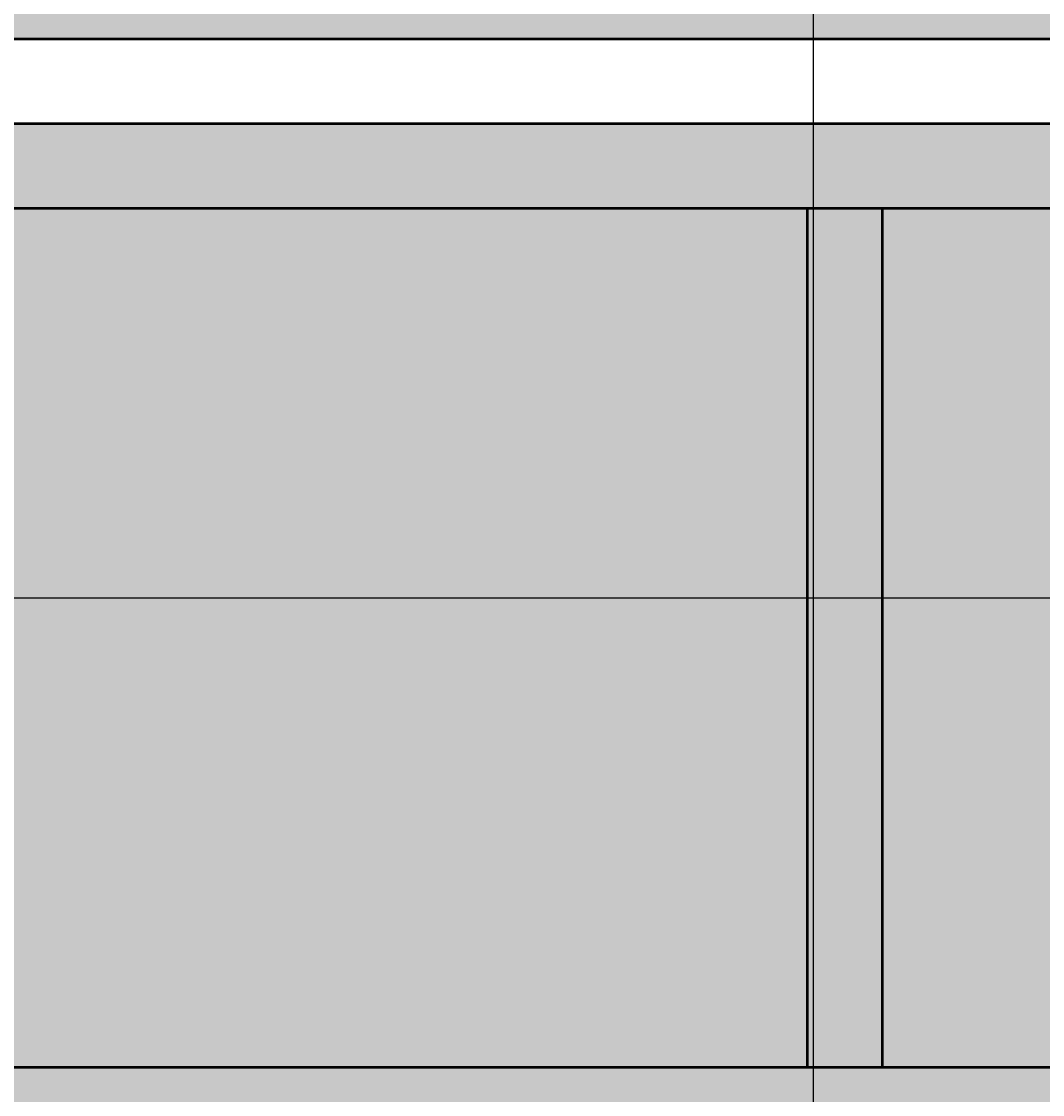
# Model space of a CAD drawing. Units: inches. Extents: x -12 to 334, y -10 to 186.
# Tile 52 of 77: x 198 to 222, y 69 to 94. Entities that reach past the tile are written whole.
import ezdxf

# ---------------------------------------------------------------- set-up
doc = ezdxf.new("R2010")
doc.units = ezdxf.units.IN
doc.header["$MEASUREMENT"] = 0
for name, color, linetype, lineweight in [('M-DIMS', 2, 'Continuous', 18), ('M-EQPM', 7, 'Continuous', 50), ('M-EQPM-PATT', 8, 'Continuous', 18)]:
    doc.layers.add(name, color=color, linetype=linetype, lineweight=lineweight)
doc.styles.get("Standard").update_dxf_attribs({"font": 'arial.ttf'})
doc.dimstyles.get("Standard").update_dxf_attribs({"dimtxt": 0.18, "dimasz": 0.18, "dimexe": 0.18, "dimexo": 0.0625, "dimgap": 0.09, "dimtad": 0, "dimtih": 1, "dimtoh": 1, "dimdec": 4, "dimzin": 0, "dimdsep": 46, "dimtxsty": 'Standard', "dimcen": 0.09, "dimadec": 0, "dimazin": 0, "dimtfac": 1, "dimtdec": 4, "dimtofl": 0, "dimtmove": 0, "dimatfit": 3, "dimfxl": 1, "dimtolj": 1, "dimtzin": 0, "dimarcsym": 0})

# ---------------------------------------------------------------- blocks, each defined once
blk = doc.blocks.new('*D1')
at = {"layer": 'Defpoints', "color": 0, "transparency": 16777216}
for p in [(281.426, 91.899), (3.376, 80.692), (281.426, 14.304)]:
    blk.add_point(p, dxfattribs=at)
at = {"layer": 'M-DIMS', "color": 0, "lineweight": -2, "transparency": 16777216}
for p, q in [((281.426, 91.836), (281.426, 14.124)), ((3.376, 80.629), (3.376, 14.124)), ((3.556, 14.304), (141.935, 14.304)), ((281.246, 14.304), (142.867, 14.304))]:
    blk.add_line(p, q, dxfattribs=at)
at = {"layer": 'M-DIMS', "color": 0, "transparency": 16777216}
for points in [[(3.556, 14.334), (3.556, 14.274), (3.376, 14.304)], [(281.246, 14.334), (281.246, 14.274), (281.426, 14.304)]]:
    blk.add_solid(points, dxfattribs=at)
at = {"layer": 'M-DIMS', "color": 0, "transparency": 16777216, "insert": (142.401, 14.304), "char_height": 0.18, "attachment_point": 5}
blk.add_mtext('\\A1;278.05', dxfattribs=at)
blk = doc.blocks.new('*D17')
at = {"layer": 'Defpoints', "color": 0, "transparency": 16777216}
for p in [(106.177, 102.896), (105.892, 56.321), (295.976, 56.321)]:
    blk.add_point(p, dxfattribs=at)
at = {"layer": 'M-DIMS', "color": 0, "lineweight": -2, "transparency": 16777216}
for p, q in [((106.24, 102.896), (296.156, 102.896)), ((295.976, 102.716), (295.976, 79.79)), ((295.976, 56.501), (295.976, 79.426)), ((105.954, 56.321), (296.156, 56.321))]:
    blk.add_line(p, q, dxfattribs=at)
at = {"layer": 'M-DIMS', "color": 0, "transparency": 16777216}
for points in [[(295.946, 102.716), (296.006, 102.716), (295.976, 102.896)], [(295.946, 56.501), (296.006, 56.501), (295.976, 56.321)]]:
    blk.add_solid(points, dxfattribs=at)
at = {"layer": 'M-DIMS', "color": 0, "transparency": 16777216, "insert": (295.976, 79.608), "char_height": 0.18, "attachment_point": 5}
blk.add_mtext('\\A1;46.575', dxfattribs=at)
blk = doc.blocks.new('*D27')
at = {"layer": 'Defpoints', "color": 0, "transparency": 16777216}
for p in [(238.576, 169.385), (216.576, 32.854), (238.576, 32.854)]:
    blk.add_point(p, dxfattribs=at)
at = {"layer": 'M-DIMS', "color": 0, "lineweight": -2, "transparency": 16777216}
for p, q in [((216.576, 32.917), (216.576, 169.565)), ((216.756, 169.385), (227.357, 169.385)), ((238.396, 169.385), (227.796, 169.385)), ((238.576, 32.917), (238.576, 169.565))]:
    blk.add_line(p, q, dxfattribs=at)
at = {"layer": 'M-DIMS', "color": 0, "transparency": 16777216}
for points in [[(216.756, 169.415), (216.756, 169.355), (216.576, 169.385)], [(238.396, 169.415), (238.396, 169.355), (238.576, 169.385)]]:
    blk.add_solid(points, dxfattribs=at)
at = {"layer": 'M-DIMS', "color": 0, "transparency": 16777216, "insert": (227.576, 169.385), "char_height": 0.18, "attachment_point": 5}
blk.add_mtext('\\A1;22', dxfattribs=at)
blk = doc.blocks.new('*D33')
at = {"layer": 'Defpoints', "color": 0, "transparency": 16777216}
for p in [(226.608, 79.754), (216.428, 61.105), (226.608, 14.304)]:
    blk.add_point(p, dxfattribs=at)
at = {"layer": 'M-DIMS', "color": 0, "lineweight": -2, "transparency": 16777216}
for p, q in [((226.608, 79.692), (226.608, 14.124)), ((216.428, 61.042), (216.428, 14.124)), ((216.608, 14.304), (221.133, 14.304)), ((226.428, 14.304), (221.903, 14.304))]:
    blk.add_line(p, q, dxfattribs=at)
at = {"layer": 'M-DIMS', "color": 0, "transparency": 16777216}
for points in [[(216.608, 14.334), (216.608, 14.274), (216.428, 14.304)], [(226.428, 14.334), (226.428, 14.274), (226.608, 14.304)]]:
    blk.add_solid(points, dxfattribs=at)
at = {"layer": 'M-DIMS', "color": 0, "transparency": 16777216, "insert": (221.518, 14.304), "char_height": 0.18, "attachment_point": 5}
blk.add_mtext('\\A1;10.18', dxfattribs=at)
blk = doc.blocks.new('*D35')
at = {"layer": 'Defpoints', "color": 0, "transparency": 16777216}
for p in [(216.428, 98.108), (-11.174, 61.105), (216.428, 61.105)]:
    blk.add_point(p, dxfattribs=at)
at = {"layer": 'M-DIMS', "color": 0, "lineweight": -2, "transparency": 16777216}
for p, q in [((216.365, 98.108), (-11.354, 98.108)), ((-11.174, 97.928), (-11.174, 79.788)), ((-11.174, 61.285), (-11.174, 79.424)), ((216.365, 61.105), (-11.354, 61.105))]:
    blk.add_line(p, q, dxfattribs=at)
at = {"layer": 'M-DIMS', "color": 0, "transparency": 16777216}
for points in [[(-11.204, 97.928), (-11.144, 97.928), (-11.174, 98.108)], [(-11.204, 61.285), (-11.144, 61.285), (-11.174, 61.105)]]:
    blk.add_solid(points, dxfattribs=at)
at = {"layer": 'M-DIMS', "color": 0, "transparency": 16777216, "insert": (-11.174, 79.606), "char_height": 0.18, "attachment_point": 5}
blk.add_mtext('\\A1;37', dxfattribs=at)
blk = doc.blocks.new('*D39')
at = {"layer": 'Defpoints', "color": 0, "transparency": 16777216}
for p in [(279.726, 80.692), (-11.174, 45.854), (269.381, 45.854)]:
    blk.add_point(p, dxfattribs=at)
at = {"layer": 'M-DIMS', "color": 0, "lineweight": -2, "transparency": 16777216}
for p, q in [((279.664, 80.692), (-11.354, 80.692)), ((-11.174, 80.512), (-11.174, 63.455)), ((-11.174, 46.034), (-11.174, 63.091)), ((269.318, 45.854), (-11.354, 45.854))]:
    blk.add_line(p, q, dxfattribs=at)
at = {"layer": 'M-DIMS', "color": 0, "transparency": 16777216}
for points in [[(-11.204, 80.512), (-11.144, 80.512), (-11.174, 80.692)], [(-11.204, 46.034), (-11.144, 46.034), (-11.174, 45.854)]]:
    blk.add_solid(points, dxfattribs=at)
at = {"layer": 'M-DIMS', "color": 0, "transparency": 16777216, "insert": (-11.174, 63.273), "char_height": 0.18, "attachment_point": 5}
blk.add_mtext('\\A1;34.84', dxfattribs=at)
blk = doc.blocks.new('*D40')
at = {"layer": 'Defpoints', "color": 0, "transparency": 16777216}
for p in [(278.229, 116.208), (187.394, 91.899)]:
    blk.add_point(p, dxfattribs=at)
at = {"layer": 'M-DIMS', "color": 0, "lineweight": -2, "transparency": 16777216}
for p, q in [((332.73, 130.793), (278.403, 116.254)), ((187.304, 91.899), (187.484, 91.899)), ((187.394, 91.809), (187.394, 91.989))]:
    blk.add_line(p, q, dxfattribs=at)
at = {"layer": 'M-DIMS', "color": 0, "transparency": 16777216}
blk.add_solid([(278.395, 116.283), (278.411, 116.225), (278.229, 116.208)], dxfattribs=at)
at = {"layer": 'M-DIMS', "color": 0, "transparency": 16777216, "insert": (333.21, 130.793), "char_height": 0.18, "attachment_point": 5}
blk.add_mtext('\\A1;R94.03', dxfattribs=at)
blk = doc.blocks.new('*D41')
at = {"layer": 'Defpoints', "color": 0, "transparency": 16777216}
for p in [(190.169, 91.899), (277.343, 68.515)]:
    blk.add_point(p, dxfattribs=at)
at = {"layer": 'M-DIMS', "color": 0, "lineweight": -2, "transparency": 16777216}
for p, q in [((190.079, 91.899), (190.259, 91.899)), ((190.169, 91.809), (190.169, 91.989)), ((329.648, 54.485), (277.517, 68.469)), ((329.828, 54.485), (329.648, 54.485))]:
    blk.add_line(p, q, dxfattribs=at)
at = {"layer": 'M-DIMS', "color": 0, "transparency": 16777216}
blk.add_solid([(277.525, 68.498), (277.509, 68.44), (277.343, 68.515)], dxfattribs=at)
at = {"layer": 'M-DIMS', "color": 0, "transparency": 16777216, "insert": (330.307, 54.485), "char_height": 0.18, "attachment_point": 5}
blk.add_mtext('\\A1;R90.26', dxfattribs=at)

msp = doc.modelspace()

# ---------------------------------------------------------------- hatches: boundary and pattern name
at = {"layer": 'M-EQPM-PATT'}
h = msp.add_hatch(color=256, dxfattribs=at)
h.set_gradient(color1=(205, 32, 39), color2=(205, 32, 39), tint=1)
h.paths.add_polyline_path([(64.5, 80.754), (64.5, 89.8963), (226.6083, 89.8963, -1), (226.6083, 69.6117), (64.5, 69.6117), (64.5, 78.754), (4.4744, 78.754, 0.384914), (23.5807, 61.4872), (37.1002, 61.4872), (37.1002, 33.6752), (53.1002, 33.6752), (53.1002, 61.4872), (64.5, 61.4872), (64.5, 63.6117), (226.6083, 63.6117, 1), (226.6083, 95.8963), (64.5, 95.8963), (64.5, 99.8958), (53.1002, 99.8958), (53.1002, 127.7078), (37.1002, 127.7078), (37.1002, 99.8958), (23.5807, 99.8958, 0.4132606), (4.3766, 80.754)])
h.paths.add_polyline_path([(64.5, 91.8963), (64.5, 93.8963), (226.6083, 93.8963, -1), (226.6083, 65.6117), (64.5, 65.6117), (64.5, 67.6117), (226.6083, 67.6117, 1), (226.6083, 91.8963)], flags=16)
h = msp.add_hatch(color=256, dxfattribs=at)
h.set_gradient(color1=(99, 100, 102), color2=(99, 100, 102), tint=1)
h.paths.add_polyline_path([(72.9244, 95.8963), (75.9244, 95.8963), (75.9244, 109.0583), (72.9244, 109.0583)])
h.paths.add_polyline_path([(72.9244, 50.4497), (75.9244, 50.4497), (75.9244, 63.6117), (72.9244, 63.6117)])
h.paths.add_polyline_path([(75.9244, 91.8963), (75.9244, 93.8963), (72.9244, 93.8963), (72.9244, 91.8963)])
h.paths.add_polyline_path([(75.9244, 65.6117), (75.9244, 67.6117), (72.9244, 67.6117), (72.9244, 65.6117)])
h.paths.add_polyline_path([(129.093, 69.6117), (130.8573, 69.6117), (130.8573, 89.8963), (129.093, 89.8963)])
h.paths.add_polyline_path([(129.093, 98.1081), (129.093, 95.8963), (130.8573, 95.8963), (130.8573, 98.1081)])
h.paths.add_polyline_path([(130.8573, 61.1045), (130.8573, 63.6117), (129.093, 63.6117), (129.093, 61.1045)])
h.paths.add_polyline_path([(170.9079, 69.6117), (172.6722, 69.6117), (172.6722, 89.8963), (170.9079, 89.8963)])
h.paths.add_polyline_path([(172.6722, 95.8963), (172.6722, 98.1081), (170.9079, 98.1081), (170.9079, 95.8963)])
h.paths.add_polyline_path([(170.9079, 61.1045), (172.6722, 61.1045), (172.6722, 63.6117), (170.9079, 63.6117)])
h.paths.add_polyline_path([(218.1922, 63.6117), (216.4278, 63.6117), (216.4278, 61.1045), (218.1922, 61.1045)])
h.paths.add_polyline_path([(216.4278, 69.6117), (218.1922, 69.6117), (218.1922, 89.8963), (216.4278, 89.8963)])
h.paths.add_polyline_path([(216.4278, 95.8963), (218.1922, 95.8963), (218.1922, 98.1081), (216.4278, 98.1081)])
h = msp.add_hatch(color=256, dxfattribs=at)
h.set_gradient(color1=(94, 103, 175), color2=(94, 103, 175), tint=1)
h.paths.add_polyline_path([(129.093, 89.8963), (86.8879, 89.8963), (86.8879, 69.6117), (129.093, 69.6117)], flags=17)
h.paths.add_polyline_path([(170.9079, 89.8963), (130.8573, 89.8963), (130.8573, 69.6117), (170.9079, 69.6117)], flags=17)
h.paths.add_polyline_path([(216.4278, 89.8963), (172.6722, 89.8963), (172.6722, 69.6117), (216.4278, 69.6117)], flags=17)
h.paths.add_polyline_path([(245.9354, 82.6969), (247.9354, 82.6969), (247.9354, 46.8541), (268.3808, 46.8541, 0.0998398), (279.7263, 80.6915), (251.9801, 80.6915, 0.4142136), (231.7758, 100.8958), (84.7229, 100.8958), (84.7229, 109.0583), (83.7229, 109.0583), (83.7229, 95.8963), (129.093, 95.8963), (129.093, 98.1081), (130.8573, 98.1081), (130.8573, 95.8963), (170.9079, 95.8963), (170.9079, 98.1081), (172.6722, 98.1081), (172.6722, 95.8963), (216.4278, 95.8963), (216.4278, 98.1081), (218.1922, 98.1081), (218.1922, 95.8963), (226.6083, 95.8963, -1), (226.6083, 63.6117), (218.1922, 63.6117), (218.1922, 61.1045), (216.4278, 61.1045), (216.4278, 63.6117), (172.6722, 63.6117), (172.6722, 61.1045), (170.9079, 61.1045), (170.9079, 63.6117), (130.8573, 63.6117), (130.8573, 61.1045), (129.093, 61.1045), (129.093, 63.6117), (87.8879, 63.6117), (87.8879, 56.3205), (105.8919, 56.3205), (105.8919, 28.8541), (115.8919, 28.8541), (115.8919, 46.8541), (222.5761, 46.8541), (222.5761, 30.8541), (232.5761, 30.8541), (232.5761, 46.8541), (245.9354, 46.8541)])
h.paths.add_polyline_path([(86.8879, 89.8963), (75.9244, 89.8963), (75.9244, 69.6117), (86.8879, 69.6117)])
h.paths.add_polyline_path([(83.7229, 109.0583), (75.9244, 109.0583), (75.9244, 95.8963), (83.7229, 95.8963)])
h.paths.add_polyline_path([(226.6083, 89.8963), (218.1922, 89.8963), (218.1922, 69.6117), (226.6083, 69.6117, 1)], flags=17)

# ---------------------------------------------------------------- linework, layer by layer
at = {"layer": 'M-EQPM'}
for points in [[(64.5, 65.6117), (226.6083, 65.6117, 1), (226.6083, 93.8963), (64.5, 93.8963)], [(64.5, 67.6117), (226.6083, 67.6117, 1), (226.6083, 91.8963), (64.5, 91.8963)], [(64.5, 69.6117), (226.6083, 69.6117, 1), (226.6083, 89.8963), (64.5, 89.8963)]]:
    msp.add_lwpolyline(points, format="xyb", dxfattribs=at)
for points in [[(216.4278, 69.6117), (216.4278, 89.8963)], [(218.1922, 89.8963), (218.1922, 69.6117)]]:
    msp.add_lwpolyline(points, dxfattribs=at)

# ---------------------------------------------------------------- dimensions: what is measured, and where the dimension line sits
at = {"layer": 'M-DIMS'}
for base, p1, p2, override, picture, middle in [((238.5761, 169.3845), (216.5761, 32.8541), (238.5761, 32.8541), {"dimdec": 0, "dimlfac": 1, "dimrnd": 0, "dimzin": 0, "dimdsep": 46, "dimlunit": 2}, '*D27', (227.5761, 169.3845)), ((281.4256, 14.3041), (3.3765, 80.6915), (281.4256, 91.8988), {"dimdec": 2, "dimlfac": 1, "dimrnd": 0, "dimzin": 0, "dimdsep": 46, "dimlunit": 2}, '*D1', (142.401, 14.3041)), ((226.6083, 14.3041), (216.4278, 61.1045), (226.6083, 79.754), {"dimdec": 2, "dimlfac": 1, "dimrnd": 0, "dimzin": 0, "dimdsep": 46, "dimlunit": 2}, '*D33', (221.5181, 14.3041))]:
    dim = msp.add_linear_dim(base=base, p1=p1, p2=p2, dimstyle='Standard', override=override, dxfattribs=at)
    dim.commit()
    dim.dimension.update_dxf_attribs({"geometry": picture, "text_midpoint": middle})
for center, mpoint, picture, middle in [((187.3936, 91.8988), (278.2291, 116.2078), '*D40', (332.7304, 130.7932)), ((190.1689, 91.8988), (277.3431, 68.5153), '*D41', (330.3074, 54.4851))]:
    dim = msp.add_radius_dim(center=center, mpoint=mpoint, dimstyle='Standard', override={"dimdec": 2, "dimlfac": 1, "dimrnd": 0, "dimzin": 0, "dimdsep": 46, "dimlunit": 2}, dxfattribs=at)
    dim.commit()
    dim.dimension.update_dxf_attribs({"geometry": picture, "text_midpoint": middle, "dimtype": 164})
for base, p1, p2, override, picture, middle in [((295.9756, 56.3205), (106.1771, 102.8958), (105.8919, 56.3205), {"dimdec": 3, "dimlfac": 1, "dimrnd": 0, "dimzin": 0, "dimdsep": 46, "dimlunit": 2}, '*D17', (295.9756, 79.6082)), ((-11.1736, 61.1045), (216.4278, 98.1081), (216.4278, 61.1045), {"dimdec": 0, "dimlfac": 1, "dimrnd": 0, "dimzin": 0, "dimdsep": 46, "dimlunit": 2}, '*D35', (-11.1735, 79.6063)), ((-11.1736, 45.8541), (279.7263, 80.6915), (269.3808, 45.8541), {"dimdec": 2, "dimlfac": 1, "dimrnd": 0, "dimzin": 0, "dimdsep": 46, "dimlunit": 2}, '*D39', (-11.1735, 63.2728))]:
    dim = msp.add_linear_dim(base=base, p1=p1, p2=p2, angle=90, dimstyle='Standard', override=override, dxfattribs=at)
    dim.commit()
    dim.dimension.update_dxf_attribs({"geometry": picture, "text_midpoint": middle})

doc.saveas('drawing.dxf')
